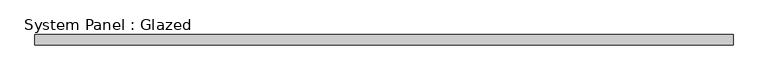
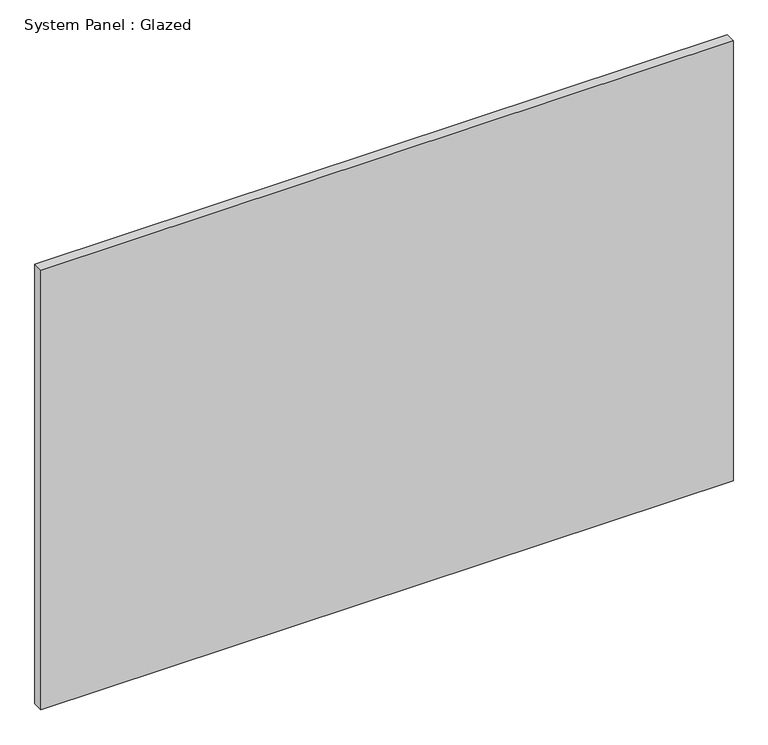
"""IFC4 building model written with IfcOpenShell, lengths in millimetres: plate geometry, System Panel : Glazed."""

from ifc_helpers import new_model, si_unit, origin, origin_with_axes, place, context, project, spatial, polyline, outline, extrude, source, transform, mapped, element, save


def system_panel_glazed_8dce6023(model_context):
    return source(origin(), model_context, "Body", "SweptSolid", [
        extrude(outline(polyline([(860.4662548, 19.05), (-860.4662548, 19.05), (-860.4662548, 44.45), (860.4662548, 44.45), (860.4662548, 19.05)])), origin_with_axes(), (0.0, 0.0, 1.0), 1155.7),
    ])


if __name__ == "__main__":
    model = new_model("IFC4")
    model_context = context("Model", 3, world=origin())
    ifc_project = project(units=[si_unit("LENGTHUNIT", "METRE", prefix="MILLI")], contexts=[model_context])
    site = spatial("IfcSite", under=ifc_project)
    building = spatial("IfcBuilding", under=site)
    placement = place(None, origin())
    system_panel_glazed_shape = system_panel_glazed_8dce6023(model_context)
    element("IfcPlate", 1, ObjectType="System Panel : Glazed", at=placement, inside=building, context=model_context, shape_type="MappedRepresentation", body=[
        mapped(system_panel_glazed_shape, transform((0.0, 0.0, 0.0), x_axis=(1.0, 0.0, 0.0), y_axis=(0.0, 1.0, 0.0), z_axis=(0.0, 0.0, 1.0))),
    ])
    save(model, "model.ifc")

# Revit data of these elements
# Type "System Panel : Glazed"
#   Construction Type Id = "GSP4R"
#   Analytic Construction = "1/8 in Pilkington single glazing"
#   Visual Light Transmittance = 0.9
#   Solar Heat Gain Coefficient = 0.86
#   Heat Transfer Coefficient (U) = 1.18115 BTU/(h·ft²·°F)
# Element 1 (IfcPlate, "System Panel : Glazed")
#   Materials on its faces: "Glass"
# Materials
#   "Glass": class "Glass", colour RGB 0 128 192, transparency 0.75, Description = "Soda Lime Glass", Cost = 0
